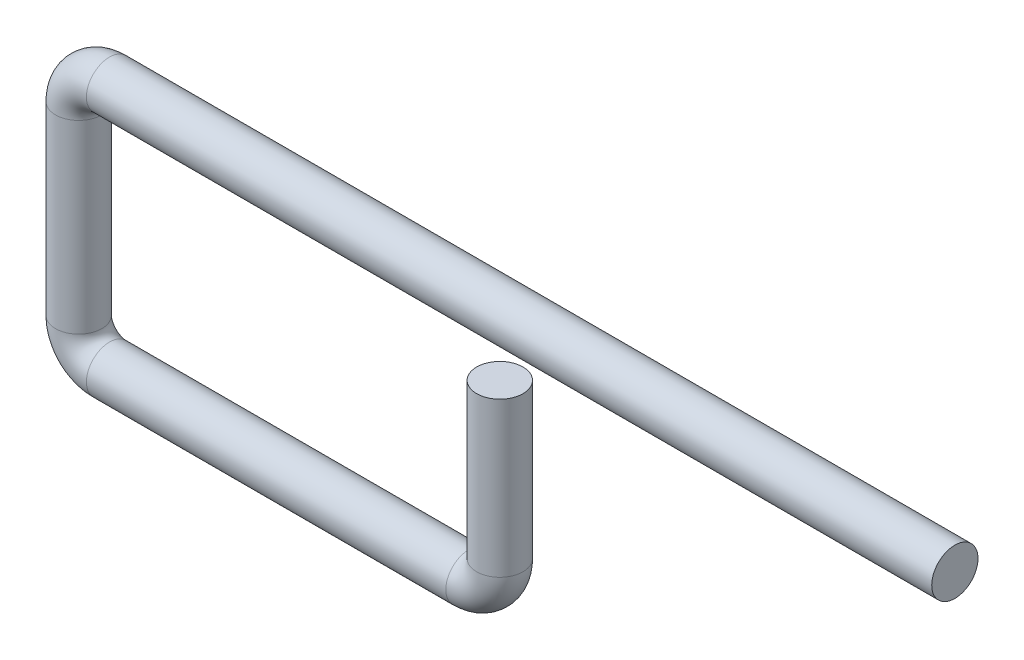
ISO-10303-21;
HEADER;
FILE_DESCRIPTION(('STEP AP214'),'2;1');
FILE_NAME('part.step','',(''),(''),'','','');
FILE_SCHEMA(('AUTOMOTIVE_DESIGN { 1 0 10303 214 1 1 1 1 }'));
ENDSEC;
DATA;
#1=APPLICATION_CONTEXT('core data for automotive mechanical design processes');
#2=APPLICATION_PROTOCOL_DEFINITION('international standard','automotive_design',2000,#1);
#3=PRODUCT_CONTEXT('',#1,'mechanical');
#4=PRODUCT('Part','Part','',(#3));
#5=PRODUCT_RELATED_PRODUCT_CATEGORY('part','',(#4));
#6=PRODUCT_DEFINITION_FORMATION('','',#4);
#7=PRODUCT_DEFINITION_CONTEXT('part definition',#1,'design');
#8=PRODUCT_DEFINITION('design','',#6,#7);
#9=PRODUCT_DEFINITION_SHAPE('','',#8);
#10=(LENGTH_UNIT() NAMED_UNIT(*) SI_UNIT(.MILLI.,.METRE.));
#11=(NAMED_UNIT(*) PLANE_ANGLE_UNIT() SI_UNIT($,.RADIAN.));
#12=(NAMED_UNIT(*) SI_UNIT($,.STERADIAN.) SOLID_ANGLE_UNIT());
#13=UNCERTAINTY_MEASURE_WITH_UNIT(LENGTH_MEASURE(1.E-05),#10,'distance_accuracy_value','');
#14=(GEOMETRIC_REPRESENTATION_CONTEXT(3) GLOBAL_UNCERTAINTY_ASSIGNED_CONTEXT((#13)) GLOBAL_UNIT_ASSIGNED_CONTEXT((#10,
#11,#12)) REPRESENTATION_CONTEXT('',''));
#15=CARTESIAN_POINT('',(0.,0.,0.));
#16=DIRECTION('',(0.,0.,1.));
#17=DIRECTION('',(1.,0.,0.));
#18=AXIS2_PLACEMENT_3D('',#15,#16,#17);
#19=CARTESIAN_POINT('',(0.,0.,0.));
#20=DIRECTION('',(0.,1.,0.));
#21=DIRECTION('',(-1.,0.,0.));
#22=AXIS2_PLACEMENT_3D('',#19,#20,#21);
#23=PLANE('',#22);
#24=CARTESIAN_POINT('',(0.,0.,0.));
#25=DIRECTION('',(0.,1.,0.));
#26=DIRECTION('',(-1.,0.,0.));
#27=AXIS2_PLACEMENT_3D('',#24,#25,#26);
#28=CIRCLE('',#27,3.75);
#29=CARTESIAN_POINT('',(-3.75,0.,0.));
#30=VERTEX_POINT('',#29);
#31=EDGE_CURVE('E80',#30,#30,#28,.T.);
#32=ORIENTED_EDGE('',*,*,#31,.T.);
#33=EDGE_LOOP('',(#32));
#34=FACE_BOUND('',#33,.T.);
#35=ADVANCED_FACE('F47',(#34),#23,.T.);
#36=CARTESIAN_POINT('',(73.75,9.99999999999999,0.));
#37=DIRECTION('',(-1.,0.,0.));
#38=DIRECTION('',(0.,-1.,0.));
#39=AXIS2_PLACEMENT_3D('',#36,#37,#38);
#40=PLANE('',#39);
#41=CARTESIAN_POINT('',(73.75,9.99999999999999,0.));
#42=DIRECTION('',(-1.,0.,0.));
#43=DIRECTION('',(0.,-1.,0.));
#44=AXIS2_PLACEMENT_3D('',#41,#42,#43);
#45=CIRCLE('',#44,3.75);
#46=CARTESIAN_POINT('',(73.75,6.24999999999999,0.));
#47=VERTEX_POINT('',#46);
#48=EDGE_CURVE('E11',#47,#47,#45,.T.);
#49=ORIENTED_EDGE('',*,*,#48,.F.);
#50=EDGE_LOOP('',(#49));
#51=FACE_BOUND('',#50,.T.);
#52=ADVANCED_FACE('F84',(#51),#40,.F.);
#53=CARTESIAN_POINT('',(0.,0.,0.));
#54=DIRECTION('',(0.,-1.,0.));
#55=DIRECTION('',(1.,0.,0.));
#56=AXIS2_PLACEMENT_3D('',#53,#54,#55);
#57=CYLINDRICAL_SURFACE('',#56,3.75);
#58=CARTESIAN_POINT('',(0.,-25.,0.));
#59=DIRECTION('',(0.,1.,0.));
#60=DIRECTION('',(-1.,0.,0.));
#61=AXIS2_PLACEMENT_3D('',#58,#59,#60);
#62=CIRCLE('',#61,3.75);
#63=CARTESIAN_POINT('',(3.75,-24.9999999999999,0.));
#64=VERTEX_POINT('',#63);
#65=EDGE_CURVE('E74',#64,#64,#62,.T.);
#66=ORIENTED_EDGE('',*,*,#65,.T.);
#67=EDGE_LOOP('',(#66));
#68=FACE_BOUND('',#67,.T.);
#69=ORIENTED_EDGE('',*,*,#31,.F.);
#70=EDGE_LOOP('',(#69));
#71=FACE_BOUND('',#70,.T.);
#72=ADVANCED_FACE('F85',(#68,#71),#57,.T.);
#73=CARTESIAN_POINT('',(-5.,-25.,0.));
#74=DIRECTION('',(0.,0.,-1.));
#75=DIRECTION('',(-1.,0.,0.));
#76=AXIS2_PLACEMENT_3D('',#73,#74,#75);
#77=TOROIDAL_SURFACE('',#76,5.,3.75);
#78=CARTESIAN_POINT('',(-5.00000000000003,-30.,0.));
#79=DIRECTION('',(1.,0.,0.));
#80=DIRECTION('',(0.,1.,0.));
#81=AXIS2_PLACEMENT_3D('',#78,#79,#80);
#82=CIRCLE('',#81,3.75);
#83=CARTESIAN_POINT('',(-5.00000000000006,-33.75,0.));
#84=VERTEX_POINT('',#83);
#85=EDGE_CURVE('E72',#84,#84,#82,.T.);
#86=CARTESIAN_POINT('',(-5.,-25.,0.));
#87=DIRECTION('',(0.,0.,-1.));
#88=DIRECTION('',(-1.,0.,0.));
#89=AXIS2_PLACEMENT_3D('',#86,#87,#88);
#90=CIRCLE('',#89,8.75);
#91=EDGE_CURVE('',#64,#84,#90,.T.);
#92=ORIENTED_EDGE('',*,*,#65,.F.);
#93=ORIENTED_EDGE('',*,*,#85,.T.);
#94=ORIENTED_EDGE('',*,*,#91,.T.);
#95=ORIENTED_EDGE('',*,*,#91,.F.);
#96=EDGE_LOOP('',(#92,#94,#93,#95));
#97=FACE_BOUND('',#96,.T.);
#98=ADVANCED_FACE('F82',(#97),#77,.T.);
#99=CARTESIAN_POINT('',(-5.00000000000003,-30.,0.));
#100=DIRECTION('',(-1.,0.,0.));
#101=DIRECTION('',(0.,-1.,0.));
#102=AXIS2_PLACEMENT_3D('',#99,#100,#101);
#103=CYLINDRICAL_SURFACE('',#102,3.75);
#104=CARTESIAN_POINT('',(-63.25,-30.,0.));
#105=DIRECTION('',(1.,0.,0.));
#106=DIRECTION('',(0.,1.,0.));
#107=AXIS2_PLACEMENT_3D('',#104,#105,#106);
#108=CIRCLE('',#107,3.75);
#109=CARTESIAN_POINT('',(-63.2499999999999,-33.75,0.));
#110=VERTEX_POINT('',#109);
#111=EDGE_CURVE('E68',#110,#110,#108,.T.);
#112=ORIENTED_EDGE('',*,*,#111,.T.);
#113=EDGE_LOOP('',(#112));
#114=FACE_BOUND('',#113,.T.);
#115=ORIENTED_EDGE('',*,*,#85,.F.);
#116=EDGE_LOOP('',(#115));
#117=FACE_BOUND('',#116,.T.);
#118=ADVANCED_FACE('F95',(#114,#117),#103,.T.);
#119=CARTESIAN_POINT('',(-63.25,-25.,0.));
#120=DIRECTION('',(0.,0.,-1.));
#121=DIRECTION('',(-1.,0.,0.));
#122=AXIS2_PLACEMENT_3D('',#119,#120,#121);
#123=TOROIDAL_SURFACE('',#122,5.,3.75);
#124=CARTESIAN_POINT('',(-68.25,-25.,0.));
#125=DIRECTION('',(0.,-1.,0.));
#126=DIRECTION('',(1.,0.,0.));
#127=AXIS2_PLACEMENT_3D('',#124,#125,#126);
#128=CIRCLE('',#127,3.75);
#129=CARTESIAN_POINT('',(-72.,-25.,0.));
#130=VERTEX_POINT('',#129);
#131=EDGE_CURVE('E62',#130,#130,#128,.T.);
#132=CARTESIAN_POINT('',(-63.25,-25.,0.));
#133=DIRECTION('',(0.,0.,-1.));
#134=DIRECTION('',(-1.,0.,0.));
#135=AXIS2_PLACEMENT_3D('',#132,#133,#134);
#136=CIRCLE('',#135,8.75);
#137=EDGE_CURVE('',#110,#130,#136,.T.);
#138=ORIENTED_EDGE('',*,*,#111,.F.);
#139=ORIENTED_EDGE('',*,*,#131,.T.);
#140=ORIENTED_EDGE('',*,*,#137,.T.);
#141=ORIENTED_EDGE('',*,*,#137,.F.);
#142=EDGE_LOOP('',(#138,#140,#139,#141));
#143=FACE_BOUND('',#142,.T.);
#144=ADVANCED_FACE('F108',(#143),#123,.T.);
#145=CARTESIAN_POINT('',(-68.25,-25.,0.));
#146=DIRECTION('',(0.,1.,0.));
#147=DIRECTION('',(0.,0.,1.));
#148=AXIS2_PLACEMENT_3D('',#145,#146,#147);
#149=CYLINDRICAL_SURFACE('',#148,3.75);
#150=CARTESIAN_POINT('',(-68.25,4.99999999999996,0.));
#151=DIRECTION('',(0.,-1.,0.));
#152=DIRECTION('',(1.,0.,0.));
#153=AXIS2_PLACEMENT_3D('',#150,#151,#152);
#154=CIRCLE('',#153,3.75);
#155=CARTESIAN_POINT('',(-72.,4.99999999999994,0.));
#156=VERTEX_POINT('',#155);
#157=EDGE_CURVE('E56',#156,#156,#154,.T.);
#158=ORIENTED_EDGE('',*,*,#157,.T.);
#159=EDGE_LOOP('',(#158));
#160=FACE_BOUND('',#159,.T.);
#161=ORIENTED_EDGE('',*,*,#131,.F.);
#162=EDGE_LOOP('',(#161));
#163=FACE_BOUND('',#162,.T.);
#164=ADVANCED_FACE('F103',(#160,#163),#149,.T.);
#165=CARTESIAN_POINT('',(-63.25,5.,0.));
#166=DIRECTION('',(0.,0.,-1.));
#167=DIRECTION('',(-1.,0.,0.));
#168=AXIS2_PLACEMENT_3D('',#165,#166,#167);
#169=TOROIDAL_SURFACE('',#168,5.,3.75);
#170=CARTESIAN_POINT('',(-63.25,10.0000000000004,0.));
#171=DIRECTION('',(-1.,0.,0.));
#172=DIRECTION('',(0.,-1.,0.));
#173=AXIS2_PLACEMENT_3D('',#170,#171,#172);
#174=CIRCLE('',#173,3.75);
#175=CARTESIAN_POINT('',(-63.25,13.75,0.));
#176=VERTEX_POINT('',#175);
#177=EDGE_CURVE('E54',#176,#176,#174,.T.);
#178=CARTESIAN_POINT('',(-63.25,5.,0.));
#179=DIRECTION('',(0.,0.,-1.));
#180=DIRECTION('',(-1.,0.,0.));
#181=AXIS2_PLACEMENT_3D('',#178,#179,#180);
#182=CIRCLE('',#181,8.75);
#183=EDGE_CURVE('',#156,#176,#182,.T.);
#184=ORIENTED_EDGE('',*,*,#157,.F.);
#185=ORIENTED_EDGE('',*,*,#177,.T.);
#186=ORIENTED_EDGE('',*,*,#183,.T.);
#187=ORIENTED_EDGE('',*,*,#183,.F.);
#188=EDGE_LOOP('',(#184,#186,#185,#187));
#189=FACE_BOUND('',#188,.T.);
#190=ADVANCED_FACE('F98',(#189),#169,.T.);
#191=CARTESIAN_POINT('',(-63.25,9.99999999999999,0.));
#192=DIRECTION('',(1.,0.,0.));
#193=DIRECTION('',(0.,1.,0.));
#194=AXIS2_PLACEMENT_3D('',#191,#192,#193);
#195=CYLINDRICAL_SURFACE('',#194,3.75);
#196=ORIENTED_EDGE('',*,*,#48,.T.);
#197=EDGE_LOOP('',(#196));
#198=FACE_BOUND('',#197,.T.);
#199=ORIENTED_EDGE('',*,*,#177,.F.);
#200=EDGE_LOOP('',(#199));
#201=FACE_BOUND('',#200,.T.);
#202=ADVANCED_FACE('F96',(#198,#201),#195,.T.);
#203=CLOSED_SHELL('',(#35,#52,#72,#98,#118,#144,#164,#190,#202));
#204=MANIFOLD_SOLID_BREP('B2',#203);
#205=ADVANCED_BREP_SHAPE_REPRESENTATION('',(#18,#204),#14);
#206=SHAPE_DEFINITION_REPRESENTATION(#9,#205);
ENDSEC;
END-ISO-10303-21;
